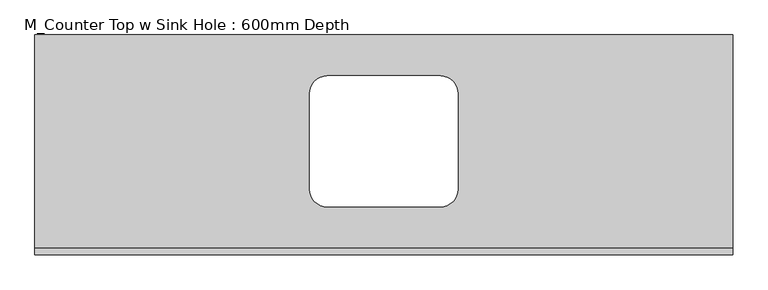
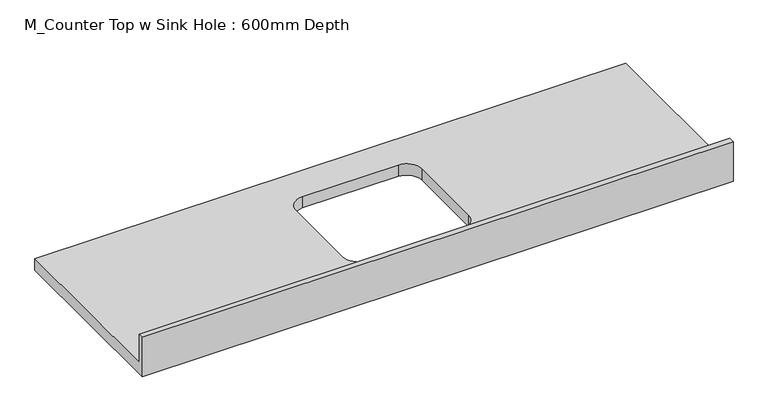
"""IFC4 building model written with IfcOpenShell, lengths in millimetres: furniture geometry, M_Counter Top w Sink Hole : 600mm Depth."""

from ifc_helpers import new_model, si_unit, frame, origin, place, context, project, spatial, polyline, circle_curve, source, transform, mapped, element, save
from ifc_brep_helpers import plane_surface, revolved_surface, advanced_brep


def m_counter_top_w_sink_hole_600mm_depth_2c7d9717(model_context):
    return source(origin(), model_context, "Body", "AdvancedBrep", [
        advanced_brep(
        [(-1200.4622951, 630.0, 900.0), (-1200.4622951, 19.05, 900.0), (799.5377049, 19.05, 900.0), (799.5377049, 630.0, 900.0), (-362.3622951, 137.3, 900.0), (-413.1622951, 188.1, 900.0), (-413.1622951, 461.9, 900.0), (-362.3622951, 512.7, 900.0), (-38.5622951, 512.7, 900.0), (12.2377049, 461.9, 900.0), (12.2377049, 188.1, 900.0), (-38.5622951, 137.3, 900.0), (799.5377049, 0.0, 860.0), (-1200.4622951, 0.0, 860.0), (-1200.4622951, 630.0, 860.0), (799.5377049, 630.0, 860.0), (-38.5622951, 137.3, 860.0), (12.2377049, 188.1, 860.0), (12.2377049, 461.9, 860.0), (-38.5622951, 512.7, 860.0), (-362.3622951, 512.7, 860.0), (-413.1622951, 461.9, 860.0), (-413.1622951, 188.1, 860.0), (-362.3622951, 137.3, 860.0), (799.5377049, 0.0, 1001.6), (-1200.4622951, 0.0, 1001.6), (-1200.4622951, 19.05, 1001.6), (799.5377049, 19.05, 1001.6)],
        [
            (0, 1),
            (1, 2),
            (2, 3),
            (3, 0),
            (4, 5, circle_curve(frame((-362.3622951, 188.1, 900.0), z_axis=(0.0, 0.0, -1.0), x_axis=(1.0, 0.0, 0.0)), 50.8)),
            (5, 6),
            (6, 7, circle_curve(frame((-362.3622951, 461.9, 900.0), z_axis=(0.0, 0.0, -1.0), x_axis=(1.0, 0.0, 0.0)), 50.8)),
            (7, 8),
            (8, 9, circle_curve(frame((-38.5622951, 461.9, 900.0), z_axis=(0.0, 0.0, -1.0), x_axis=(1.0, 0.0, 0.0)), 50.8)),
            (9, 10),
            (10, 11, circle_curve(frame((-38.5622951, 188.1, 900.0), z_axis=(0.0, 0.0, -1.0), x_axis=(1.0, 0.0, 0.0)), 50.8)),
            (11, 4),
            (12, 13),
            (13, 14),
            (14, 15),
            (15, 12),
            (16, 17, circle_curve(frame((-38.5622951, 188.1, 860.0), z_axis=(0.0, 0.0, 1.0), x_axis=(1.0, 0.0, 0.0)), 50.8)),
            (17, 18),
            (18, 19, circle_curve(frame((-38.5622951, 461.9, 860.0), z_axis=(0.0, 0.0, 1.0), x_axis=(1.0, 0.0, 0.0)), 50.8)),
            (19, 20),
            (20, 21, circle_curve(frame((-362.3622951, 461.9, 860.0), z_axis=(0.0, 0.0, 1.0), x_axis=(1.0, 0.0, 0.0)), 50.8)),
            (21, 22),
            (22, 23, circle_curve(frame((-362.3622951, 188.1, 860.0), z_axis=(0.0, 0.0, 1.0), x_axis=(1.0, 0.0, 0.0)), 50.8)),
            (23, 16),
            (12, 24),
            (24, 25),
            (25, 13),
            (25, 26),
            (26, 1),
            (0, 14),
            (3, 15),
            (2, 27),
            (27, 24),
            (27, 26),
            (11, 16),
            (23, 4),
            (22, 5),
            (21, 6),
            (20, 7),
            (19, 8),
            (18, 9),
            (17, 10),
        ],
        [
            plane_surface(frame((-1200.4622951, 0.0, 900.0), z_axis=(0.0, 0.0, 1.0), x_axis=(-1.0, 0.0, 0.0))),
            plane_surface(frame((-1200.4622951, 0.0, 860.0), z_axis=(0.0, 0.0, -1.0), x_axis=(1.0, 0.0, 0.0))),
            plane_surface(frame((799.5377049, 0.0, 900.0), z_axis=(0.0, -1.0, 0.0), x_axis=(0.0, 0.0, -1.0))),
            plane_surface(frame((-1200.4622951, 0.0, 900.0), z_axis=(-1.0, 0.0, 0.0), x_axis=(0.0, 0.0, -1.0))),
            plane_surface(frame((-1200.4622951, 630.0, 900.0), z_axis=(0.0, 1.0, 0.0), x_axis=(0.0, 0.0, -1.0))),
            plane_surface(frame((799.5377049, 630.0, 900.0), z_axis=(1.0, 0.0, 0.0), x_axis=(0.0, 0.0, -1.0))),
            plane_surface(frame((-1200.4622951, 0.0, 1001.6), z_axis=(0.0, 0.0, 1.0), x_axis=(0.0, 1.0, 0.0))),
            plane_surface(frame((-1200.4622951, 19.05, 1001.6), z_axis=(0.0, 1.0, 0.0), x_axis=(0.0, 0.0, -1.0))),
            plane_surface(frame((-38.5622951, 137.3, 900.0), z_axis=(0.0, 1.0, 0.0), x_axis=(0.0, 0.0, -1.0))),
            revolved_surface(polyline([(-311.5622951, 188.1, 900.0), (-311.5622951, 188.1, 860.0)]), (-362.3622951, 188.1, 860.0), (0.0, 0.0, 1.0)),
            plane_surface(frame((-413.1622951, 188.1, 900.0), z_axis=(1.0, 0.0, 0.0), x_axis=(0.0, 0.0, -1.0))),
            revolved_surface(polyline([(-311.5622951, 461.9, 900.0), (-311.5622951, 461.9, 860.0)]), (-362.3622951, 461.9, 860.0), (0.0, 0.0, 1.0)),
            plane_surface(frame((-362.3622951, 512.7, 900.0), z_axis=(0.0, -1.0, 0.0), x_axis=(0.0, 0.0, -1.0))),
            revolved_surface(polyline([(12.237704899999997, 461.9, 900.0), (12.237704899999997, 461.9, 860.0)]), (-38.5622951, 461.9, 860.0), (0.0, 0.0, 1.0)),
            plane_surface(frame((12.2377049, 461.9, 900.0), z_axis=(-1.0, 0.0, 0.0), x_axis=(0.0, 0.0, -1.0))),
            revolved_surface(polyline([(12.237704899999997, 188.1, 900.0), (12.237704899999997, 188.1, 860.0)]), (-38.5622951, 188.1, 860.0), (0.0, 0.0, 1.0)),
        ],
        [
            (0, [[1, 2, 3, 4], [5, 6, 7, 8, 9, 10, 11, 12]]),
            (1, [[13, 14, 15, 16], [17, 18, 19, 20, 21, 22, 23, 24]]),
            (2, [[25, 26, 27, -13]]),
            (3, [[-27, 28, 29, -1, 30, -14]]),
            (4, [[31, -15, -30, -4]]),
            (5, [[-31, -3, 32, 33, -25, -16]]),
            (6, [[-26, -33, 34, -28]]),
            (7, [[-32, -2, -29, -34]]),
            (8, [[-12, 35, -24, 36]]),
            (9, [[-23, 37, -5, -36]]),
            (10, [[-22, 38, -6, -37]]),
            (11, [[-21, 39, -7, -38]]),
            (12, [[-20, 40, -8, -39]]),
            (13, [[-19, 41, -9, -40]]),
            (14, [[-18, 42, -10, -41]]),
            (15, [[-11, -42, -17, -35]]),
        ],
    ),
    ])


if __name__ == "__main__":
    model = new_model("IFC4")
    model_context = context("Model", 3, world=origin())
    ifc_project = project(units=[si_unit("LENGTHUNIT", "METRE", prefix="MILLI")], contexts=[model_context])
    site = spatial("IfcSite", under=ifc_project)
    building = spatial("IfcBuilding", under=site)
    placement = place(None, origin())
    m_counter_top_w_sink_hole_600mm_depth_shape = m_counter_top_w_sink_hole_600mm_depth_2c7d9717(model_context)
    element("IfcFurniture", 1, ObjectType="M_Counter Top w Sink Hole : 600mm Depth", at=placement, inside=building, context=model_context, shape_type="MappedRepresentation", body=[
        mapped(m_counter_top_w_sink_hole_600mm_depth_shape, transform((0.0, 0.0, 0.0), x_axis=(1.0, 0.0, 0.0), y_axis=(0.0, 1.0, 0.0), z_axis=(0.0, 0.0, 1.0))),
    ])
    save(model, "model.ifc")

# Revit data of these elements
# Type "M_Counter Top w Sink Hole : 600mm Depth"
#   Counter Thickness = 0.131234 ft
#   Depth [instance default] = 2.050525 ft
#   Height = 2.952756 ft
#   Length [instance default] = 8.2021 ft
#   Sink Location [instance default] = 3.937008 ft
#   Sink Location To Wall [instance default] = 0.328084 ft
#   Sink Opening Depth [instance default] = 1.240157 ft
#   Sink Opening Width [instance default] = 1.925853 ft
#   Counter Top Material = none
#   Default Elevation = 0
# Element 1 (IfcFurniture, "M_Counter Top w Sink Hole : 600mm Depth")
#   Depth = 2.066929 ft
#   Length = 6.56168 ft
#   Sink Location = 3.28084 ft
#   Sink Location To Wall = 0.492126 ft
#   Sink Opening Depth = 1.148294 ft
#   Sink Opening Width = 1.312336 ft
#   Materials on its faces: "Counter Top"
# Materials
#   "Counter Top": class "Wood", colour RGB 226 177 128, transparency 0
